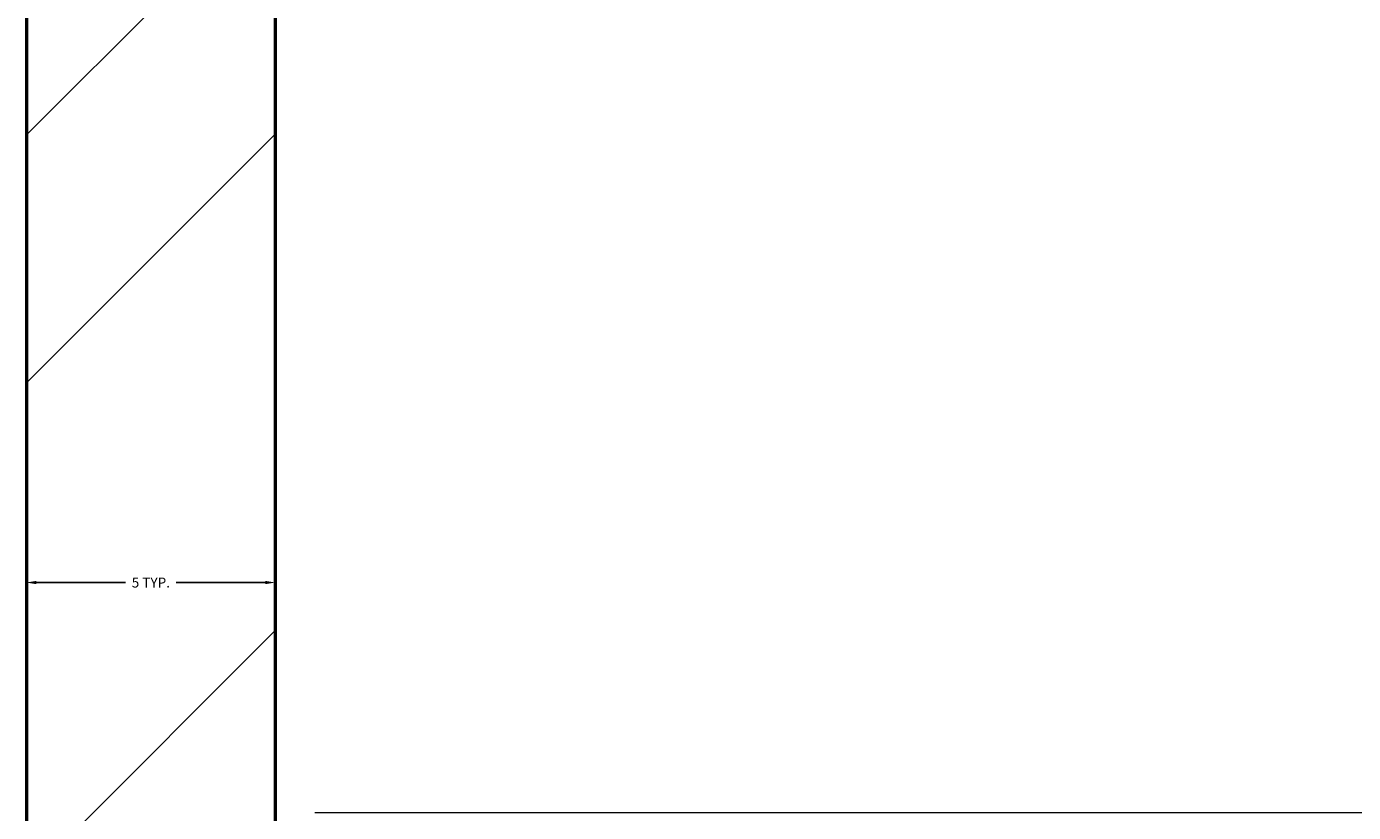
# Model space of a CAD drawing. Units: inches. Extents: x 1901 to 2863, y 888 to 2433.
# Tile 58 of 91: x 2025 to 2049, y 2188 to 2202. Entities that reach past the tile are written whole.
import ezdxf

# ---------------------------------------------------------------- set-up
doc = ezdxf.new("R2010")
doc.units = ezdxf.units.IN
for name, color, linetype, lineweight in [('A-ANNO-DIMS', 2, 'Continuous', 18), ('A-FURN', 8, 'Continuous', 18), ('A-WALL', 7, 'Continuous', 50), ('A-WALL-PATT', 8, 'Continuous', 13)]:
    doc.layers.add(name, color=color, linetype=linetype, lineweight=lineweight)
doc.styles.get("Standard").update_dxf_attribs({"font": 'arial.ttf'})
doc.dimstyles.get("Standard").update_dxf_attribs({"dimtxt": 0.18, "dimasz": 0.18, "dimexe": 0.18, "dimexo": 0.0625, "dimgap": 0.09, "dimtad": 0, "dimtih": 1, "dimtoh": 1, "dimdec": 4, "dimzin": 0, "dimdsep": 46, "dimtxsty": 'Standard', "dimcen": 0.09, "dimadec": 0, "dimazin": 0, "dimtfac": 1, "dimtdec": 4, "dimtofl": 0, "dimtmove": 0, "dimatfit": 3, "dimfxl": 1, "dimtolj": 1, "dimtzin": 0, "dimarcsym": 0})

# ---------------------------------------------------------------- blocks, each defined once
blk = doc.blocks.new('BED-DOUBLE')
blk.add_line((0.744, 57.778), (30.62, 57.778))
blk = doc.blocks.new('*D22')
at = {"layer": 'A-ANNO-DIMS', "color": 0, "lineweight": -2, "transparency": 16777216}
for p, q in [((2024.926, 2184.802), (2024.926, 2192.119)), ((2029.426, 2184.802), (2029.426, 2192.119)), ((2025.106, 2191.939), (2026.718, 2191.939)), ((2029.246, 2191.939), (2027.634, 2191.939))]:
    blk.add_line(p, q, dxfattribs=at)
at = {"layer": 'A-ANNO-DIMS', "color": 0, "transparency": 16777216}
for points in [[(2025.106, 2191.969), (2025.106, 2191.909), (2024.926, 2191.939)], [(2029.246, 2191.969), (2029.246, 2191.909), (2029.426, 2191.939)]]:
    blk.add_solid(points, dxfattribs=at)
at = {"layer": 'Defpoints', "color": 0, "transparency": 16777216}
for p in [(2024.926, 2191.939), (2024.926, 2184.739), (2029.426, 2184.739)]:
    blk.add_point(p, dxfattribs=at)
at = {"layer": 'A-ANNO-DIMS', "color": 0, "transparency": 16777216, "insert": (2027.176, 2191.939), "char_height": 0.18, "attachment_point": 5}
blk.add_mtext('\\A1;5 TYP.', dxfattribs=at)

msp = doc.modelspace()

# ---------------------------------------------------------------- hatches: boundary and pattern name
at = {"layer": 'A-WALL-PATT'}
h = msp.add_hatch(dxfattribs=at)
h.set_pattern_fill('ANSI32', color=256)
h.paths.add_polyline_path([(2192.501, 2274.134), (2141.264, 2274.134), (2141.264, 2269.634), (2192.501, 2269.634)])
h.paths.add_polyline_path([(2259.926, 2274.134), (2216.501, 2274.134), (2216.501, 2269.634), (2255.426, 2269.634), (2255.426, 2214.634), (2250.809, 2214.634), (2250.809, 2210.134), (2259.926, 2210.134), (2259.926, 2215.134), (2271.756, 2215.134), (2271.756, 2217.384), (2271.756, 2219.634), (2259.926, 2219.634)])
h.paths.add_polyline_path([(2171.426, 2269.634), (2166.926, 2269.634), (2166.926, 2219.634), (2121.238, 2219.634), (2121.238, 2215.134), (2166.926, 2215.134), (2166.926, 2083.134), (2161.807, 2083.134), (2161.807, 2078.634), (2171.426, 2078.634), (2176.996, 2078.634), (2176.996, 2080.884), (2176.996, 2083.134), (2171.426, 2083.134), (2171.426, 2210.134), (2230.912, 2210.134), (2230.912, 2212.384), (2230.912, 2214.634), (2171.426, 2214.634)])
h.paths.add_polyline_path([(2117.264, 2274.134), (2089.426, 2274.134), (2089.426, 2219.634), (2081.136, 2219.634), (2081.136, 2215.134), (2089.426, 2215.134), (2098.004, 2215.134), (2098.004, 2217.384), (2098.004, 2219.634), (2093.926, 2219.634), (2093.926, 2269.634), (2117.264, 2269.634), (2117.264, 2271.884)])
h.paths.add_polyline_path([(2343.426, 2219.634), (2329.295, 2219.634), (2329.295, 2215.134), (2338.926, 2215.134), (2338.926, 2184.739), (2343.426, 2184.739)])
h.paths.add_polyline_path([(2338.926, 2083.134), (2329.295, 2083.134), (2208.966, 2083.134), (2208.966, 2078.634), (2338.926, 2078.634)])
h.paths.add_polyline_path([(2343.426, 2136.739), (2338.926, 2136.739), (2338.926, 1872.634), (2343.426, 1872.634)])
h.paths.add_polyline_path([(2343.426, 1863.634), (2397.68, 1863.634), (2397.68, 1821.634), (2384.138, 1821.634), (2384.138, 1812.634), (2418.33, 1812.634), (2418.33, 1817.134), (2418.33, 1821.634), (2406.68, 1821.634), (2406.68, 1863.634), (2459.499, 1863.634), (2459.499, 1821.634), (2447.138, 1821.634), (2447.138, 1812.634), (2459.499, 1812.634), (2468.499, 1812.634), (2468.499, 1872.634), (2394.426, 1872.634), (2334.426, 1872.634), (2334.426, 1812.634), (2343.426, 1812.634), (2353.251, 1812.634), (2353.251, 1821.634), (2343.426, 1821.634)])
h.paths.add_polyline_path([(2510.014, 1872.634), (2468.499, 1872.634), (2468.499, 1868.134), (2510.014, 1868.134)])
h.paths.add_polyline_path([(2514.009, 1817.134), (2468.499, 1817.134), (2468.499, 1812.634), (2482.114, 1812.634), (2482.114, 1800.606), (2486.614, 1800.606), (2486.614, 1812.634), (2514.009, 1812.634)])
h.paths.add_polyline_path([(2299.247, 1814.884), (2299.247, 1817.134), (2295.926, 1817.134), (2295.926, 1854.169), (2293.676, 1854.169), (2291.426, 1854.169), (2291.426, 1817.134), (2266.109, 1817.134), (2266.109, 1812.634), (2299.247, 1812.634)])
h.paths.add_polyline_path([(2218.109, 1817.134), (2206.46, 1817.134), (2171.426, 1817.134), (2171.426, 1949.134), (2190.1, 1949.134), (2190.1, 1953.634), (2163.468, 1953.634), (2163.468, 1949.134), (2166.926, 1949.134), (2166.926, 1817.134), (2114.297, 1817.134), (2114.297, 1812.634), (2218.109, 1812.634)])
h.paths.add_polyline_path([(2029.426, 1970.922), (2024.926, 1970.922), (2024.926, 1912.717), (2029.426, 1912.717)])
h.paths.add_polyline_path([(2132.297, 1953.634), (2113.926, 1953.634), (2113.926, 1975.888), (2111.676, 1975.888), (2109.426, 1975.888), (2109.426, 1953.634), (2029.426, 1953.634), (2029.426, 1949.134), (2132.297, 1949.134)])
h.paths.add_polyline_path([(2029.426, 1853.606), (2029.31, 1853.606), (2029.31, 1853.606), (2029.426, 1853.606), (2029.426, 1864.717), (2024.926, 1864.717), (2024.926, 1812.634), (2066.297, 1812.634), (2066.297, 1814.884), (2066.297, 1817.134), (2029.426, 1817.134)])
h.paths.add_polyline_path([(2122.926, 2010.088), (2120.676, 2010.088), (2118.426, 2010.088), (2118.426, 2006.134), (2029.426, 2006.134), (2029.426, 2001.634), (2109.426, 2001.634), (2109.426, 1998.041), (2113.926, 1998.041), (2113.926, 2001.634), (2122.926, 2001.634)])
h.paths.add_polyline_path([(2029.426, 2031.376), (2024.926, 2031.376), (2024.926, 1994.922), (2027.176, 1994.922), (2029.426, 1994.922)])
h.paths.add_polyline_path([(2029.426, 2136.739), (2024.926, 2136.739), (2024.926, 2067.376), (2027.176, 2067.376), (2029.426, 2067.376)])
h.paths.add_polyline_path([(2125.618, 2083.134), (2029.426, 2083.134), (2029.426, 2078.634), (2118.426, 2078.634), (2118.426, 2030.715), (2122.926, 2030.715), (2122.926, 2078.634), (2125.618, 2078.634)])
h.paths.add_polyline_path([(2029.426, 2215.134), (2040.468, 2215.134), (2040.468, 2217.384), (2040.468, 2219.634), (2024.926, 2219.634), (2024.926, 2184.739), (2029.426, 2184.739), (2029.426, 2187.778)])
h.paths.add_polyline_path([(2686.426, 2274.134), (2659.284, 2274.134), (2659.284, 2269.634), (2681.926, 2269.634), (2681.926, 2219.634), (2676.816, 2219.634), (2676.816, 2215.134), (2681.926, 2215.134), (2697.011, 2215.134), (2697.011, 2217.384), (2697.011, 2219.634), (2686.426, 2219.634)])
h.paths.add_polyline_path([(2609.926, 2269.634), (2635.284, 2269.634), (2635.284, 2274.134), (2571.431, 2274.134), (2571.431, 2269.634), (2605.426, 2269.634), (2605.426, 2214.634), (2549.098, 2214.634), (2549.098, 2210.134), (2605.426, 2210.134), (2605.426, 2083.134), (2601.014, 2083.134), (2601.014, 2080.884), (2601.014, 2078.634), (2609.926, 2078.634), (2616.162, 2078.634), (2616.162, 2080.884), (2616.162, 2083.134), (2609.926, 2083.134), (2609.926, 2215.134), (2651.465, 2215.134), (2651.465, 2217.384), (2651.465, 2219.634), (2609.926, 2219.634)])
h.paths.add_polyline_path([(2521.426, 2269.634), (2547.431, 2269.634), (2547.431, 2271.884), (2547.431, 2274.134), (2516.926, 2274.134), (2516.926, 2219.634), (2506.41, 2219.634), (2506.41, 2215.134), (2516.926, 2215.134), (2516.926, 2210.134), (2525.402, 2210.134), (2525.402, 2212.384), (2525.402, 2214.634), (2521.426, 2214.634)])
h.paths.add_polyline_path([(2456.011, 2219.634), (2439.426, 2219.634), (2439.426, 2187.888), (2443.926, 2187.888), (2443.926, 2215.134), (2456.011, 2215.134)])
h.paths.add_polyline_path([(2752.926, 2219.634), (2739.485, 2219.634), (2739.485, 2215.134), (2748.426, 2215.134), (2748.426, 2187.888), (2752.926, 2187.888)])
h.paths.add_polyline_path([(2752.926, 2139.888), (2748.426, 2139.888), (2748.426, 2083.134), (2648.416, 2083.134), (2648.416, 2078.634), (2654.926, 2078.634), (2654.926, 2039.437), (2659.426, 2039.437), (2659.426, 2078.634), (2748.426, 2078.634), (2748.426, 2063.429), (2752.926, 2063.429)])
h.paths.add_polyline_path([(2752.926, 2010.634), (2659.426, 2010.634), (2659.426, 2015.652), (2654.926, 2015.652), (2654.926, 2010.634), (2605.426, 2010.634), (2605.426, 1920.967), (2609.926, 1920.967), (2609.926, 2006.134), (2748.426, 2006.134), (2748.426, 1982.466), (2752.926, 1982.466)])
h.paths.add_polyline_path([(2752.926, 2027.429), (2748.426, 2027.429), (2748.426, 2010.634), (2752.926, 2010.634)])
h.paths.add_polyline_path([(2748.426, 1886.134), (2609.926, 1886.134), (2609.926, 1889.719), (2605.426, 1889.719), (2605.426, 1861.262), (2609.926, 1861.262), (2609.926, 1881.634), (2748.426, 1881.634)])
h.paths.add_polyline_path([(2456.855, 2228.831), (2498.401, 2228.831), (2498.401, 2247.488), (2456.855, 2247.488)], flags=9)
h.paths.add_polyline_path([(2038.602, 2237.418), (2080.174, 2237.418), (2080.174, 2256.075), (2038.602, 2256.075)], flags=9)
h.paths.add_polyline_path([(2292.009, 1062.394), (2539.932, 1062.394), (2539.932, 1099.487), (2292.009, 1099.487)], flags=9)
h.paths.add_polyline_path([(2424.91, 1832.253), (2448.513, 1832.253), (2448.513, 1846.678), (2424.91, 1846.678)], flags=25)
h.paths.add_polyline_path([(2359.076, 1832.253), (2382.678, 1832.253), (2382.678, 1846.678), (2359.076, 1846.678)], flags=25)
h.paths.add_polyline_path([(2352.899, 1684.802), (2367.543, 1684.802), (2367.543, 1697.167), (2352.899, 1697.167)], flags=9)
h.paths.add_polyline_path([(2079.288, 1755.826), (2169.024, 1755.826), (2169.024, 1774.372), (2079.288, 1774.372)], flags=9)
h.paths.add_polyline_path([(2404.09, 1373.857), (2404.09, 1463.593), (2385.544, 1463.593), (2385.544, 1373.857)], flags=9)
h.paths.add_polyline_path([(2268.091, 2236.371), (2309.636, 2236.371), (2309.636, 2255.028), (2268.091, 2255.028)], flags=9)
h.paths.add_polyline_path([(2575.96, 1700.951), (2665.696, 1700.951), (2665.696, 1719.498), (2575.96, 1719.498)], flags=9)
h.paths.add_polyline_path([(2302.962, 1878.474), (2329.524, 1878.474), (2329.524, 1888.777), (2302.962, 1888.777)], flags=9)
h.paths.add_polyline_path([(2097.415, 2240.576), (2126.573, 2240.576), (2126.573, 2259.233), (2097.415, 2259.233)], flags=9)
h.paths.add_polyline_path([(2208.725, 2246.124), (2237.882, 2246.124), (2237.882, 2264.781), (2208.725, 2264.781)], flags=9)
h.paths.add_polyline_path([(2038.147, 1925.958), (2076.987, 1925.958), (2076.987, 1944.615), (2038.147, 1944.615)], flags=9)
h.paths.add_polyline_path([(2239.144, 1926.672), (2288.465, 1926.672), (2288.465, 1945.329), (2239.144, 1945.329)], flags=9)
h.paths.add_polyline_path([(2175.429, 2007.33), (2212.356, 2007.33), (2212.356, 2025.987), (2175.429, 2025.987)], flags=9)
h.paths.add_polyline_path([(2225.034, 2091.794), (2263.875, 2091.794), (2263.875, 2110.451), (2225.034, 2110.451)], flags=9)
h.paths.add_polyline_path([(2035.398, 2098.478), (2074.238, 2098.478), (2074.238, 2117.135), (2035.398, 2117.135)], flags=9)
h.paths.add_polyline_path([(2050.102, 2029.209), (2083.26, 2029.209), (2083.26, 2047.866), (2050.102, 2047.866)], flags=9)
h.paths.add_polyline_path([(2069.677, 1956.719), (2098.835, 1956.719), (2098.835, 1975.376), (2069.677, 1975.376)], flags=25)
h.paths.add_polyline_path([(2328.62, 1753.336), (2361.663, 1753.336), (2361.663, 1771.993), (2328.62, 1771.993)], flags=9)
h.paths.add_polyline_path([(2395.162, 2060.888), (2395.162, 2140.654), (2378.676, 2140.654), (2378.676, 2060.888)], flags=9)
h.paths.add_polyline_path([(2463.728, 2059.02), (2492.886, 2059.02), (2492.886, 2077.677), (2463.728, 2077.677)], flags=9)
h.paths.add_polyline_path([(2458.027, 2181.536), (2496.868, 2181.536), (2496.868, 2200.194), (2458.027, 2200.194)], flags=9)
h.paths.add_polyline_path([(2527.577, 2243.074), (2556.735, 2243.074), (2556.735, 2261.731), (2527.577, 2261.731)], flags=9)
h.paths.add_polyline_path([(2694.461, 2232.767), (2736.033, 2232.767), (2736.033, 2251.425), (2694.461, 2251.425)], flags=9)
h.paths.add_polyline_path([(2637.821, 2249.225), (2666.979, 2249.225), (2666.979, 2267.882), (2637.821, 2267.882)], flags=9)
h.paths.add_polyline_path([(2623.687, 2183.541), (2662.528, 2183.541), (2662.528, 2202.199), (2623.687, 2202.199)], flags=9)
h.paths.add_polyline_path([(2691.965, 2021.5), (2725.124, 2021.5), (2725.124, 2040.157), (2691.965, 2040.157)], flags=9)
h.paths.add_polyline_path([(2621.043, 1975.912), (2662.335, 1975.912), (2662.335, 1994.569), (2621.043, 1994.569)], flags=25)
h.paths.add_polyline_path([(2479.032, 1927.62), (2519.844, 1927.62), (2519.844, 1946.277), (2479.032, 1946.277)], flags=9)
h.paths.add_polyline_path([(2670.941, 1849.076), (2716.005, 1849.076), (2716.005, 1867.734), (2670.941, 1867.734)], flags=9)
h.paths.add_polyline_path([(2523.613, 1782.956), (2550.175, 1782.956), (2550.175, 1793.26), (2523.613, 1793.26)], flags=9)
h.paths.add_polyline_path([(2450.841, 1207.331), (2492.386, 1207.331), (2492.386, 1225.989), (2450.841, 1225.989)], flags=9)
h.paths.add_polyline_path([(2527.751, 1203.841), (2556.908, 1203.841), (2556.908, 1222.499), (2527.751, 1222.499)], flags=9)
h.paths.add_polyline_path([(2639.111, 1207.2), (2668.268, 1207.2), (2668.268, 1225.857), (2639.111, 1225.857)], flags=9)
h.paths.add_polyline_path([(2692.594, 1218.965), (2734.167, 1218.965), (2734.167, 1237.623), (2692.594, 1237.623)], flags=9)
h.paths.add_polyline_path([(2669.266, 1366.329), (2708.106, 1366.329), (2708.106, 1384.987), (2669.266, 1384.987)], flags=9)
h.paths.add_polyline_path([(2463.313, 1358.031), (2502.153, 1358.031), (2502.153, 1376.688), (2463.313, 1376.688)], flags=9)
h.paths.add_polyline_path([(2494.725, 1449.963), (2531.652, 1449.963), (2531.652, 1468.62), (2494.725, 1468.62)], flags=9)
h.paths.add_polyline_path([(2675.565, 1422.157), (2708.724, 1422.157), (2708.724, 1440.815), (2675.565, 1440.815)], flags=9)
h.paths.add_polyline_path([(2685.634, 1493.891), (2714.792, 1493.891), (2714.792, 1512.548), (2685.634, 1512.548)], flags=9)
h.paths.add_polyline_path([(2686.805, 1529.913), (2725.645, 1529.913), (2725.645, 1548.57), (2686.805, 1548.57)], flags=9)
h.paths.add_polyline_path([(2503.651, 1537.991), (2552.972, 1537.991), (2552.972, 1556.648), (2503.651, 1556.648)], flags=9)
h.paths.add_polyline_path([(2291.713, 1643.504), (2318.275, 1643.504), (2318.275, 1653.807), (2291.713, 1653.807)], flags=9)
h.paths.add_polyline_path([(2450.626, 1610.52), (2477.189, 1610.52), (2477.189, 1620.824), (2450.626, 1620.824)], flags=9)
h.paths.add_polyline_path([(2359.985, 1551.814), (2422.253, 1551.814), (2422.253, 1562.117), (2359.985, 1562.117)], flags=9)
h.paths.add_polyline_path([(2280.106, 1249.006), (2321.651, 1249.006), (2321.651, 1267.663), (2280.106, 1267.663)], flags=9)
h.paths.add_polyline_path([(2164.057, 1274.232), (2193.215, 1274.232), (2193.215, 1292.889), (2164.057, 1292.889)], flags=9)
h.paths.add_polyline_path([(2118.21, 1277.694), (2151.252, 1277.694), (2151.252, 1296.351), (2118.21, 1296.351)], flags=9)
h.paths.add_polyline_path([(2031.946, 1268.529), (2073.519, 1268.529), (2073.519, 1287.187), (2031.946, 1287.187)], flags=9)
h.paths.add_polyline_path([(2050.199, 1409.079), (2089.04, 1409.079), (2089.04, 1427.736), (2050.199, 1427.736)], flags=9)
h.paths.add_polyline_path([(2243.743, 1421.032), (2282.584, 1421.032), (2282.584, 1439.689), (2243.743, 1439.689)], flags=9)
h.paths.add_polyline_path([(2190.746, 1509.769), (2231.558, 1509.769), (2231.558, 1528.426), (2190.746, 1528.426)], flags=9)
h.paths.add_polyline_path([(2058.392, 1475.415), (2091.55, 1475.415), (2091.55, 1494.073), (2058.392, 1494.073)], flags=9)
h.paths.add_polyline_path([(2062.447, 1553.09), (2091.605, 1553.09), (2091.605, 1571.747), (2062.447, 1571.747)], flags=9)
h.paths.add_polyline_path([(2219.524, 1590.365), (2266.147, 1590.365), (2266.147, 1609.022), (2219.524, 1609.022)], flags=9)
h.paths.add_polyline_path([(2041.072, 1584.188), (2079.912, 1584.188), (2079.912, 1602.845), (2041.072, 1602.845)], flags=9)

# ---------------------------------------------------------------- linework, layer by layer
at = {"layer": 'A-WALL'}
for p, q in [((2024.926, 2219.634), (2024.926, 1812.634)), ((2029.426, 2215.134), (2029.426, 1817.134))]:
    msp.add_line(p, q, dxfattribs=at)

# ---------------------------------------------------------------- block references
at = {"layer": 'A-FURN'}
msp.add_blockref('BED-DOUBLE', (2029.4, 2130), dxfattribs=at)

# ---------------------------------------------------------------- dimensions: what is measured, and where the dimension line sits
at = {"layer": 'A-ANNO-DIMS'}
dim = msp.add_linear_dim(base=(2024.926174575, 2191.939408848), p1=(2029.426174575, 2184.739408848), p2=(2024.926174575, 2184.739408848), angle=180, text='<> TYP.', dimstyle='Standard', override={"dimdec": 0, "dimlfac": 1, "dimrnd": 0, "dimzin": 0, "dimdsep": 46, "dimlunit": 2}, dxfattribs=at)
dim.commit()
dim.dimension.update_dxf_attribs({"geometry": '*D22', "text_midpoint": (2027.176174575, 2191.939408848)})

doc.saveas('drawing.dxf')
